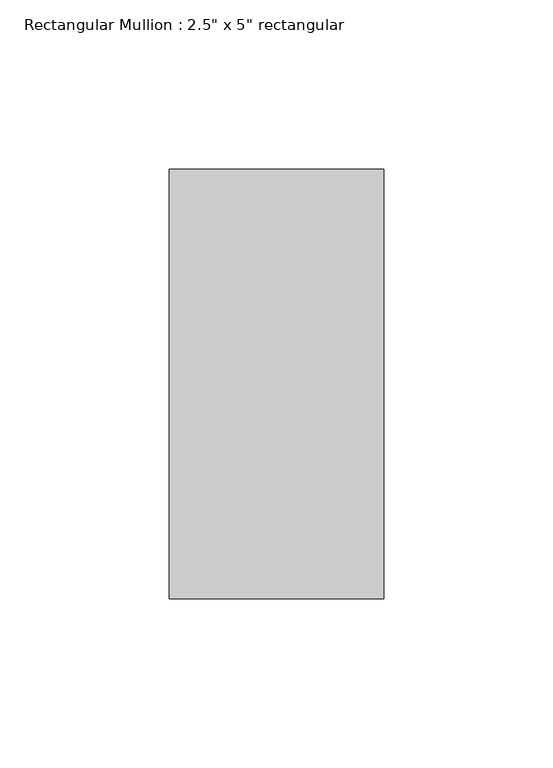
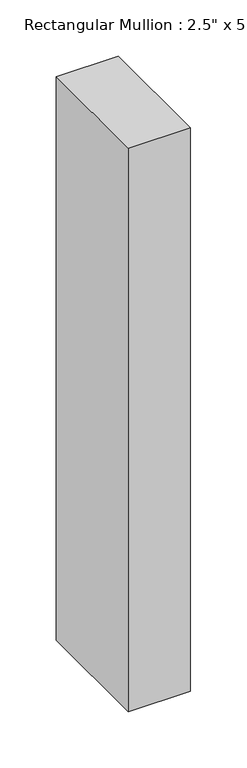
"""IFC4 building model written with IfcOpenShell, lengths in millimetres: member geometry."""

from ifc_helpers import new_model, si_unit, frame, origin, place, context, project, spatial, polyline, outline, extrude, source, transform, mapped, element, save


def member_47bfaf8a(model_context):
    return source(origin(), model_context, "Body", "SweptSolid", [
        extrude(outline(polyline([(0.0, 63.5), (0.0, -63.5), (-63.5, -63.5), (-63.5, 63.5), (0.0, 63.5)])), frame((0.0, 0.0, -609.6), z_axis=(0.0, 0.0, 1.0), x_axis=(1.0, 0.0, 0.0)), (0.0, 0.0, 1.0), 609.6),
    ])


if __name__ == "__main__":
    model = new_model("IFC4")
    model_context = context("Model", 3, world=origin())
    ifc_project = project(units=[si_unit("LENGTHUNIT", "METRE", prefix="MILLI")], contexts=[model_context])
    site = spatial("IfcSite", under=ifc_project)
    building = spatial("IfcBuilding", under=site)
    placement = place(None, origin())
    member_shape = member_47bfaf8a(model_context)
    element("IfcMember", 1, ObjectType="Rectangular Mullion : 2.5\" x 5\" rectangular", at=placement, inside=building, context=model_context, shape_type="MappedRepresentation", body=[
        mapped(member_shape, transform((0.0, 0.0, 0.0), x_axis=(1.0, 0.0, 0.0), y_axis=(0.0, 1.0, 0.0), z_axis=(0.0, 0.0, 1.0))),
    ])
    save(model, "model.ifc")

# Revit data of these elements
# Type "Rectangular Mullion : 2.5\" x 5\" rectangular"
#   built-in parameter 1007304 = 0.416667 (stored number, unit not read)
#   built-in parameter 1007301 = 0.104167 (stored number, unit not read)
#   built-in parameter 1007300 = 0.104167 (stored number, unit not read)
# Element 1 (IfcMember, "Rectangular Mullion : 2.5\" x 5\" rectangular")
#   Materials on its faces: "BLACK MATERIAL"
# Materials
#   "BLACK MATERIAL": class "Generic", colour RGB 120 120 120, transparency 0, Cost = 0
